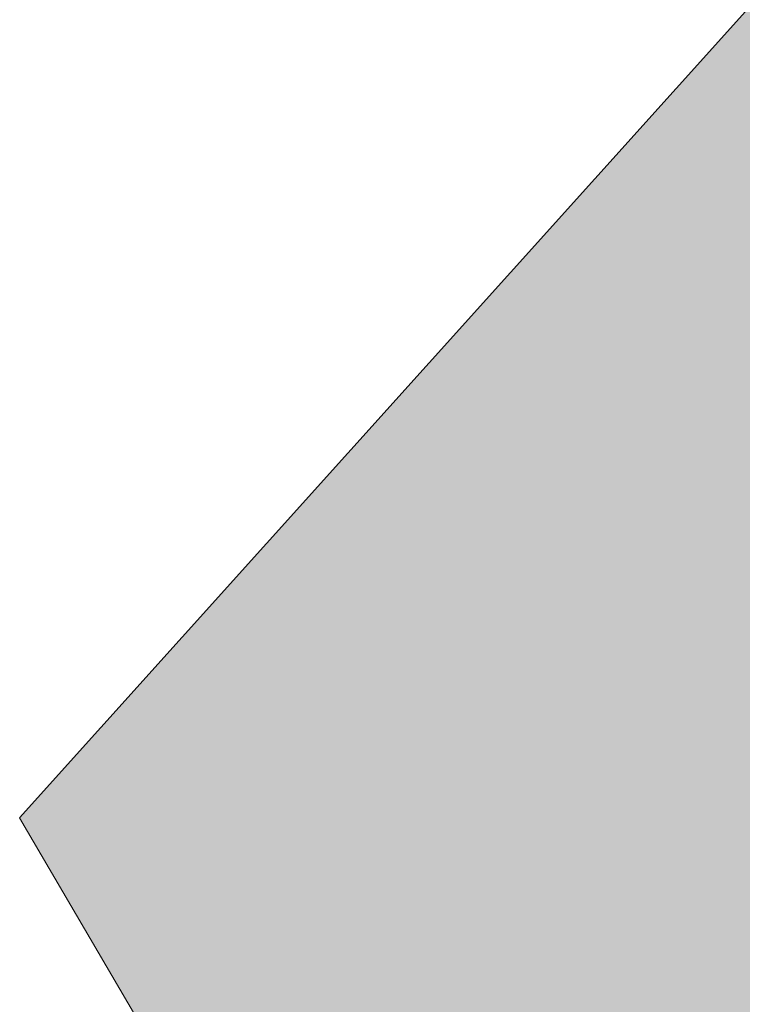
# Model space of a CAD drawing. Units: inches. Extents: x 2091 to 2899, y 967 to 2217.
# Tile 244 of 256: x 2212.563 to 2213.361, y 1135.592 to 1136.679. Entities that reach past the tile are written whole.
import ezdxf

# ---------------------------------------------------------------- set-up
doc = ezdxf.new("R2010")
doc.units = ezdxf.units.IN
doc.layers.add('L-PLNT-PATT', color=114, linetype='Continuous', lineweight=13, true_color=0x139b48)
doc.layers.add('L-PLNT-TREE', color=94, linetype='Continuous', lineweight=13)

# ---------------------------------------------------------------- blocks, each defined once
blk = doc.blocks.new('*U25')
blk.add_lwpolyline([(-1139.42368, 1783.79628), (-1216.11644, 1685.47796), (-1117.5111, 1601.2033), (-1051.7759, 1643.3419), (-1126.09884, 1521.20092), (-1072.10606, 1527.49758), (-1079.90386, 1416.93646), (-1259.93906, 1179.83508), (-1479.05978, 1165.78888), (-1577.66258, 1109.60662), (-1742.00312, 927.01364), (-1676.26538, 814.64658), (-1270.89408, 828.69278), (-1194.20386, 772.51052), (-1007.95074, 856.78518), (-876.4778, 575.87134), (-821.70016, 575.87134), (-569.71184, 884.87504)])

msp = doc.modelspace()

# ---------------------------------------------------------------- hatches: boundary and pattern name
at = {"layer": 'L-PLNT-PATT'}
h = msp.add_hatch(color=256, dxfattribs=at)
h.dxf.hatch_style = 1
h.paths.add_polyline_path([(2333.3376, 1165.6587), (2329.0242, 1166.2116), (2331.6122, 1168.4235), (2335.0629, 1177.2712), (2328.1615, 1184.4599), (2319.5348, 1187.2248), (2323.4168, 1193.3076), (2319.9661, 1203.8142), (2317.8094, 1203.8142), (2313.496, 1213.2148), (2310.908, 1212.6618), (2307.8887, 1212.6618), (2305.7319, 1217.0857), (2307.0259, 1223.1684), (2310.4767, 1223.1684), (2304.0066, 1230.9101), (2303.1363, 1237.0465), (2299.6932, 1240.8637), (2296.6739, 1237.5459), (2294.9485, 1238.6518), (2294.5171, 1241.4166), (2292.3605, 1242.5227), (2289.3411, 1239.7577), (2285.8904, 1240.3107), (2283.3024, 1235.3339), (2283.3024, 1230.9101), (2286.7531, 1229.2512), (2284.165, 1227.5922), (2281.577, 1229.8042), (2274.2442, 1222.6154), (2274.2442, 1220.9565), (2271.2249, 1219.2976), (2272.0876, 1217.6386), (2274.2442, 1214.3208), (2270.3622, 1211.5559), (2266.4801, 1214.3208), (2264.3235, 1213.7678), (2263.4608, 1211.5559), (2266.4801, 1211.0029), (2266.9115, 1206.5791), (2263.5392, 1207.132), (2259.5788, 1203.2612), (2263.8921, 1202.7082), (2262.1668, 1197.1784), (2258.2848, 1196.6254), (2253.9714, 1193.8606), (2248.7953, 1191.0957), (2248.364, 1193.3076), (2244.4819, 1185.0129), (2251.3833, 1186.6718), (2255.6967, 1183.9069), (2254.4027, 1177.2712), (2246.6387, 1174.5063), (2243.1879, 1176.7182), (2241.8939, 1173.4003), (2238.8746, 1172.8474), (2236.2865, 1169.5295), (2233.2671, 1165.6587), (2237.1492, 1162.3408), (2239.7372, 1163.9998), (2236.8111, 1159.1911), (2238.9368, 1159.439), (2238.6298, 1155.0862), (2231.5418, 1145.7515), (2222.915, 1145.1985), (2219.033, 1142.9866), (2212.5629, 1135.7979), (2215.151, 1131.374), (2231.1105, 1131.927), (2234.1298, 1129.7151), (2241.4626, 1133.033), (2246.6387, 1121.9734), (2248.7953, 1121.9734), (2258.7161, 1134.1389), (2261.7355, 1135.7979), (2263.8921, 1133.033), (2263.8921, 1129.1621), (2267.3429, 1128.0562), (2272.0876, 1128.0562), (2273.8129, 1131.927), (2279.4203, 1134.6919), (2285.0278, 1135.2449), (2287.6158, 1137.4568), (2288.0471, 1138.0098), (2289.3411, 1140.7747), (2291.0665, 1139.6687), (2292.3605, 1135.2449), (2295.3798, 1136.9038), (2296.2425, 1135.7979), (2297.1052, 1133.033), (2300.1246, 1138.0098), (2303.1439, 1138.0098), (2304.4379, 1135.7979), (2303.1439, 1133.586), (2306.5946, 1134.6919), (2307.8887, 1133.033), (2310.908, 1135.2449), (2313.9274, 1134.1389), (2319.9661, 1128.0562), (2322.5541, 1126.9502), (2324.7108, 1124.7383), (2342.827, 1126.3972), (2346.2777, 1123.0794), (2348.8658, 1124.1853), (2341.9643, 1133.033), (2341.533, 1136.3508), (2343.6897, 1139.6687), (2339.8077, 1150.1753), (2337.651, 1150.1753)])
h.paths.add_polyline_path([(2339.6578, 1120.6164), (2337.9038, 1120.3574), (2338.4438, 1119.5784), (2340.3328, 1119.6654)])
h.paths.add_polyline_path([(2341.1428, 1118.5404), (2339.0508, 1118.6264), (2339.0508, 1117.6754), (2340.9408, 1116.9824)])
h.paths.add_polyline_path([(2336.5538, 1120.8764), (2335.2038, 1120.3574), (2334.7988, 1118.9724), (2336.8238, 1119.5784)])
h.paths.add_polyline_path([(2337.2958, 1118.9724), (2336.6208, 1118.2804), (2337.6338, 1117.7614)])
h.paths.add_polyline_path([(2338.6458, 1118.7134), (2339.1858, 1119.3194), (2338.2408, 1118.8864), (2338.2408, 1118.1074)])
h.paths.add_polyline_path([(2339.0508, 1122.8664), (2337.7688, 1123.8184), (2337.0938, 1123.1254), (2337.2958, 1121.8284)])
h.paths.add_polyline_path([(2341.6148, 1122.0014), (2341.1428, 1121.8284), (2340.6708, 1122.9524), (2340.1308, 1121.8284), (2340.5358, 1121.0494), (2341.7498, 1120.5304), (2342.8298, 1121.2224)])
h.paths.add_polyline_path([(2342.9648, 1119.7514), (2342.0198, 1119.4914), (2342.0878, 1118.0214), (2343.0328, 1118.4534)])
h.paths.add_polyline_path([(2345.8668, 1118.1944), (2344.3828, 1118.6264), (2343.7078, 1118.0214), (2345.5298, 1117.3294)])
h.paths.add_polyline_path([(2344.6518, 1116.8094), (2343.6398, 1116.4634), (2343.0328, 1115.9444), (2343.9098, 1114.9064), (2344.6518, 1115.3394), (2344.1798, 1115.6854)])
h.paths.add_polyline_path([(2346.8118, 1116.9824), (2345.7318, 1115.8584), (2345.5298, 1114.1274), (2347.0138, 1112.3104), (2348.2968, 1112.2244), (2346.8798, 1114.3004), (2345.8668, 1114.2144), (2346.8118, 1114.6464)])
h.paths.add_polyline_path([(2345.2598, 1116.5504), (2344.7198, 1116.3774), (2344.9218, 1115.6854), (2345.1248, 1115.8584)])
h.paths.add_polyline_path([(2342.6948, 1116.8964), (2342.0198, 1117.3294), (2341.9528, 1116.6364)])
h.paths.add_polyline_path([(2341.4808, 1120.0974), (2341.1428, 1120.0974), (2341.0758, 1119.5784), (2341.4808, 1119.4054)])
h.paths.add_polyline_path([(2343.9778, 1121.1354), (2343.6398, 1119.7514), (2345.0568, 1119.7514)])
h.paths.add_polyline_path([(2339.1178, 1121.7414), (2338.3758, 1121.5684), (2338.1738, 1121.0494), (2338.8478, 1121.2224)])
h.paths.add_polyline_path([(2336.3508, 1122.4334), (2335.7438, 1122.7794), (2334.5288, 1123.4714), (2334.9338, 1122.4334), (2336.0138, 1121.9144)])
h.paths.add_polyline_path([(2334.4618, 1122.1744), (2332.0998, 1122.8664), (2331.3568, 1122.1744), (2332.5718, 1121.3084)])
h.paths.add_polyline_path([(2334.5968, 1121.3084), (2334.0568, 1120.7894), (2334.2588, 1120.3574), (2334.7318, 1120.8764)])
h.paths.add_polyline_path([(2332.5048, 1120.7894), (2331.6948, 1120.4434), (2332.7068, 1119.6654)])
h.paths.add_polyline_path([(2333.6518, 1119.3194), (2333.3818, 1118.4534), (2334.2588, 1118.5404)])
h.paths.add_polyline_path([(2331.9648, 1118.1944), (2331.0868, 1116.2904), (2332.6398, 1116.6364)])
h.paths.add_polyline_path([(2330.7498, 1121.5684), (2328.9948, 1121.0494), (2328.5228, 1119.3194), (2330.2768, 1120.2704)])
h.paths.add_polyline_path([(2330.7498, 1118.6264), (2329.8728, 1118.0214), (2330.0078, 1117.5024)])
h.paths.add_polyline_path([(2328.3878, 1117.8484), (2327.1728, 1117.7614), (2327.5098, 1116.5504)])
h.paths.add_polyline_path([(2326.9028, 1115.2524), (2326.0928, 1115.3394), (2325.2158, 1113.6084), (2326.7008, 1114.1274)])
h.paths.add_polyline_path([(2328.6578, 1114.3874), (2328.3198, 1114.9064), (2328.0498, 1114.1274)])
h.paths.add_polyline_path([(2326.7008, 1112.6564), (2327.1058, 1112.1374), (2328.3198, 1112.2244)])
h.paths.add_polyline_path([(2329.5348, 1113.6084), (2328.5898, 1113.3494), (2329.0628, 1112.3104)])
h.paths.add_polyline_path([(2340.3328, 1115.3394), (2339.3878, 1115.3394), (2340.0628, 1113.6954)])
h.paths.add_polyline_path([(2340.9408, 1116.3774), (2340.8058, 1115.5124), (2342.0198, 1115.0794)])
h.paths.add_polyline_path([(2341.8178, 1114.4734), (2340.8058, 1114.5604), (2340.9408, 1113.0894)])
h.paths.add_polyline_path([(2343.0328, 1112.2244), (2342.3578, 1113.3494), (2341.5478, 1112.2244), (2342.0198, 1111.7914)])
h.paths.add_polyline_path([(2342.7628, 1113.9544), (2343.4378, 1113.0894), (2344.0448, 1113.5224)])
h.paths.add_polyline_path([(2344.7198, 1114.3874), (2344.4498, 1113.8684), (2345.1918, 1113.3494)])
h.paths.add_polyline_path([(2345.6648, 1112.3104), (2344.6518, 1112.5704), (2344.0448, 1111.9644), (2345.4618, 1111.5324)])
h.paths.add_polyline_path([(2344.3148, 1111.0124), (2342.9648, 1111.0994), (2342.9648, 1110.3204)])
h.paths.add_polyline_path([(2344.8548, 1110.0614), (2344.1128, 1109.7154), (2344.5168, 1109.2824)])
h.paths.add_polyline_path([(2346.6768, 1109.2824), (2345.8668, 1110.0614), (2346.0698, 1108.0714)])
h.paths.add_polyline_path([(2347.0138, 1110.9264), (2346.6098, 1111.1864), (2346.2718, 1110.4934)])
h.paths.add_polyline_path([(2345.8668, 1106.6864), (2344.5168, 1106.6004), (2344.9898, 1105.5624)])
h.paths.add_polyline_path([(2345.1248, 1104.6974), (2344.4498, 1104.2644), (2344.5848, 1103.7454)])
h.paths.add_polyline_path([(2343.7748, 1104.4374), (2343.4378, 1105.1294), (2342.6948, 1104.6104), (2342.6278, 1102.8804)])
h.paths.add_polyline_path([(2341.8178, 1103.8314), (2341.1428, 1103.6584), (2341.5478, 1102.8804)])
h.paths.add_polyline_path([(2342.5598, 1102.3614), (2341.9528, 1101.8414), (2342.6948, 1101.6684)])
h.paths.add_polyline_path([(2341.1428, 1101.9284), (2340.6028, 1102.3614), (2340.0628, 1101.8414), (2340.6028, 1101.2364)])
h.paths.add_polyline_path([(2336.7558, 1101.2364), (2337.3638, 1100.5434), (2339.1178, 1100.4574)])
h.paths.add_polyline_path([(2335.2718, 1103.3124), (2334.1918, 1102.6204), (2335.5418, 1102.2744)])
h.paths.add_polyline_path([(2333.9888, 1101.7554), (2333.5168, 1101.5824), (2334.7318, 1101.1494)])
h.paths.add_polyline_path([(2331.6948, 1102.9664), (2330.5468, 1102.0144), (2332.0998, 1102.3614)])
h.paths.add_polyline_path([(2329.7378, 1106.5134), (2328.2528, 1106.0814), (2329.5348, 1105.3024)])
h.paths.add_polyline_path([(2326.6328, 1108.3304), (2326.4978, 1109.1094), (2325.8908, 1108.5034), (2326.0928, 1107.3794)])
h.paths.add_polyline_path([(2240.5961, 1257.8142), (2239.5841, 1257.4682), (2238.9771, 1256.9492), (2239.8541, 1255.9112), (2240.5961, 1256.3442), (2240.1241, 1256.6902)])
h.paths.add_polyline_path([(2241.8111, 1259.1992), (2240.3271, 1259.6312), (2239.6521, 1259.0262), (2241.4741, 1258.3342)])
h.paths.add_polyline_path([(2242.7561, 1257.9872), (2241.6761, 1256.8632), (2241.4741, 1255.1322), (2242.9581, 1253.3152), (2244.2411, 1253.2292), (2242.8241, 1255.3052), (2241.8111, 1255.2192), (2242.7561, 1255.6512)])
h.paths.add_polyline_path([(2241.6091, 1253.3152), (2240.5961, 1253.5752), (2239.9891, 1252.9692), (2241.4061, 1252.5372)])
h.paths.add_polyline_path([(2240.6641, 1255.3922), (2240.3941, 1254.8732), (2241.1361, 1254.3542)])
h.paths.add_polyline_path([(2242.9581, 1251.9312), (2242.5541, 1252.1912), (2242.2161, 1251.4982)])
h.paths.add_polyline_path([(2240.2591, 1252.0172), (2238.9091, 1252.1042), (2238.9091, 1251.3252)])
h.paths.add_polyline_path([(2238.3021, 1254.3542), (2237.4921, 1253.2292), (2237.9641, 1252.7962), (2238.9771, 1253.2292)])
h.paths.add_polyline_path([(2239.9891, 1254.5272), (2238.7071, 1254.9592), (2239.3821, 1254.0942)])
h.paths.add_polyline_path([(2240.7991, 1251.0662), (2240.0571, 1250.7202), (2240.4611, 1250.2872)])
h.paths.add_polyline_path([(2241.8111, 1251.0662), (2242.0141, 1249.0762), (2242.6211, 1250.2872)])
h.paths.add_polyline_path([(2241.2041, 1257.5552), (2240.6641, 1257.3822), (2240.8661, 1256.6902), (2241.0691, 1256.8632)])
h.paths.add_polyline_path([(2238.6391, 1257.9012), (2237.9641, 1258.3342), (2237.8971, 1257.6412)])
h.paths.add_polyline_path([(2238.9091, 1260.7562), (2237.9641, 1260.4962), (2238.0321, 1259.0262), (2238.9771, 1259.4582)])
h.paths.add_polyline_path([(2239.9221, 1262.1402), (2239.5841, 1260.7562), (2241.0011, 1260.7562)])
h.paths.add_polyline_path([(2238.7741, 1262.2272), (2237.5591, 1263.0062), (2237.0871, 1262.8332), (2236.6151, 1263.9572), (2236.0751, 1262.8332), (2236.4801, 1262.0542), (2237.6941, 1261.5352)])
h.paths.add_polyline_path([(2237.4251, 1261.1022), (2237.0871, 1261.1022), (2237.0201, 1260.5832), (2237.4251, 1260.4102)])
h.paths.add_polyline_path([(2237.0871, 1259.5452), (2234.9951, 1259.6312), (2234.9951, 1258.6802), (2236.8851, 1257.9872)])
h.paths.add_polyline_path([(2236.8851, 1257.3822), (2236.7501, 1256.5172), (2237.9641, 1256.0842)])
h.paths.add_polyline_path([(2237.7621, 1255.4782), (2236.7501, 1255.5652), (2236.8851, 1254.0942)])
h.paths.add_polyline_path([(2236.2771, 1256.3442), (2235.3321, 1256.3442), (2236.0071, 1254.7002)])
h.paths.add_polyline_path([(2241.8111, 1247.6912), (2240.4611, 1247.6052), (2240.9341, 1246.5672)])
h.paths.add_polyline_path([(2239.7191, 1245.4422), (2239.3821, 1246.1342), (2238.6391, 1245.6152), (2238.5721, 1243.8852)])
h.paths.add_polyline_path([(2241.0691, 1245.7022), (2240.3941, 1245.2692), (2240.5291, 1244.7502)])
h.paths.add_polyline_path([(2237.7621, 1244.8362), (2237.0871, 1244.6632), (2237.4921, 1243.8852)])
h.paths.add_polyline_path([(2237.0871, 1242.9332), (2236.5471, 1243.3662), (2236.0071, 1242.8462), (2236.5471, 1242.2412)])
h.paths.add_polyline_path([(2238.5041, 1243.3662), (2237.8971, 1242.8462), (2238.6391, 1242.6732)])
h.paths.add_polyline_path([(2232.7001, 1242.2412), (2233.3081, 1241.5482), (2235.0621, 1241.4622)], flags=17)
h.paths.add_polyline_path([(2231.2161, 1244.3172), (2230.1361, 1243.6252), (2231.4861, 1243.2792)])
h.paths.add_polyline_path([(2229.9331, 1242.7602), (2229.4611, 1242.5872), (2230.6761, 1242.1542)])
h.paths.add_polyline_path([(2227.6391, 1243.9712), (2226.4911, 1243.0192), (2228.0441, 1243.3662)])
h.paths.add_polyline_path([(2222.5771, 1249.3352), (2222.4421, 1250.1142), (2221.8351, 1249.5082), (2222.0371, 1248.3842)])
h.paths.add_polyline_path([(2225.6821, 1247.5182), (2224.1971, 1247.0862), (2225.4791, 1246.3072)])
h.paths.add_polyline_path([(2225.4791, 1254.6132), (2224.5341, 1254.3542), (2225.0071, 1253.3152)])
h.paths.add_polyline_path([(2224.2641, 1253.2292), (2222.6451, 1253.6612), (2223.0501, 1253.1422)])
h.paths.add_polyline_path([(2222.8471, 1256.2572), (2222.0371, 1256.3442), (2221.1601, 1254.6132), (2222.6451, 1255.1322)])
h.paths.add_polyline_path([(2224.3321, 1258.8532), (2223.1171, 1258.7662), (2223.4541, 1257.5552)])
h.paths.add_polyline_path([(2226.6941, 1259.6312), (2225.8171, 1259.0262), (2225.9521, 1258.5072)])
h.paths.add_polyline_path([(2227.9091, 1259.1992), (2227.0311, 1257.2952), (2228.5841, 1257.6412)])
h.paths.add_polyline_path([(2224.2641, 1255.9112), (2223.9941, 1255.1322), (2224.6021, 1255.3922)])
h.paths.add_polyline_path([(2229.5961, 1260.3242), (2229.3261, 1259.4582), (2230.2031, 1259.5452)])
h.paths.add_polyline_path([(2228.4491, 1261.7942), (2227.6391, 1261.4482), (2228.6511, 1260.6702)])
h.paths.add_polyline_path([(2230.4061, 1263.1792), (2228.0441, 1263.8712), (2227.3011, 1263.1792), (2228.5161, 1262.3132)])
h.paths.add_polyline_path([(2232.7681, 1260.5832), (2232.4981, 1261.8812), (2231.1481, 1261.3622), (2230.7431, 1259.9772)])
h.paths.add_polyline_path([(2230.6761, 1261.8812), (2230.5411, 1262.3132), (2230.0011, 1261.7942), (2230.2031, 1261.3622)])
h.paths.add_polyline_path([(2232.2951, 1263.4382), (2231.6881, 1263.7842), (2230.4731, 1264.4762), (2230.8781, 1263.4382), (2231.9581, 1262.9192)])
h.paths.add_polyline_path([(2234.9951, 1263.8712), (2233.7131, 1264.8232), (2233.0381, 1264.1302), (2233.2401, 1262.8332)])
h.paths.add_polyline_path([(2235.0621, 1262.7462), (2234.3201, 1262.5732), (2234.1181, 1262.0542), (2234.7921, 1262.2272)])
h.paths.add_polyline_path([(2235.6021, 1261.6212), (2233.8481, 1261.3622), (2234.3881, 1260.5832), (2236.2771, 1260.6702)])
h.paths.add_polyline_path([(2235.1301, 1260.3242), (2234.1851, 1259.8912), (2234.1851, 1259.1122), (2234.5901, 1259.7182)])
h.paths.add_polyline_path([(2226.6941, 1262.5732), (2224.9391, 1262.0542), (2224.4671, 1260.3242), (2226.2211, 1261.2752)])
h.paths.add_polyline_path([(2233.2401, 1259.9772), (2232.5651, 1259.2852), (2233.5781, 1258.7662)])
h.paths.add_polyline_path([(2337.2674, 1337.8275), (2336.1874, 1336.7035), (2335.9854, 1334.9725), (2337.4694, 1333.1555), (2338.7524, 1333.0695), (2337.3354, 1335.1455), (2336.3224, 1335.0595), (2337.2674, 1335.4915)])
h.paths.add_polyline_path([(2336.3224, 1339.0395), (2334.8384, 1339.4715), (2334.1634, 1338.8665), (2335.9854, 1338.1745)])
h.paths.add_polyline_path([(2334.4334, 1341.9805), (2334.0954, 1340.5965), (2335.5124, 1340.5965)])
h.paths.add_polyline_path([(2333.2854, 1342.0675), (2332.0704, 1342.8465), (2331.5984, 1342.6735), (2331.1264, 1343.7975), (2330.5864, 1342.6735), (2330.9914, 1341.8945), (2332.2054, 1341.3755)])
h.paths.add_polyline_path([(2333.4204, 1340.5965), (2332.4754, 1340.3365), (2332.5434, 1338.8665), (2333.4884, 1339.2985)])
h.paths.add_polyline_path([(2331.9364, 1340.9425), (2331.5984, 1340.9425), (2331.5314, 1340.4235), (2331.9364, 1340.2505)])
h.paths.add_polyline_path([(2329.5734, 1342.5865), (2328.8314, 1342.4135), (2328.6294, 1341.8945), (2329.3034, 1342.0675)])
h.paths.add_polyline_path([(2329.5064, 1343.7115), (2328.2244, 1344.6635), (2327.5494, 1343.9705), (2327.7514, 1342.6735)])
h.paths.add_polyline_path([(2330.1134, 1341.4615), (2328.3594, 1341.2025), (2328.8994, 1340.4235), (2330.7884, 1340.5105)])
h.paths.add_polyline_path([(2331.5984, 1339.3855), (2329.5064, 1339.4715), (2329.5064, 1338.5205), (2331.3964, 1337.8275)])
h.paths.add_polyline_path([(2327.0094, 1341.7215), (2325.6594, 1341.2025), (2325.2544, 1339.8175), (2327.2794, 1340.4235)])
h.paths.add_polyline_path([(2326.8064, 1343.2785), (2326.1994, 1343.6245), (2324.9844, 1344.3165), (2325.3894, 1343.2785), (2326.4694, 1342.7595)])
h.paths.add_polyline_path([(2324.9174, 1343.0195), (2322.5554, 1343.7115), (2321.8124, 1343.0195), (2323.0274, 1342.1535)])
h.paths.add_polyline_path([(2321.2054, 1342.4135), (2319.4504, 1341.8945), (2318.9784, 1340.1645), (2320.7324, 1341.1155)])
h.paths.add_polyline_path([(2318.8434, 1338.6935), (2317.6284, 1338.6065), (2317.9654, 1337.3955)])
h.paths.add_polyline_path([(2322.4204, 1339.0395), (2321.5424, 1337.1355), (2323.0954, 1337.4815)])
h.paths.add_polyline_path([(2324.1074, 1340.1645), (2323.8374, 1339.2985), (2324.7144, 1339.3855)])
h.paths.add_polyline_path([(2322.9604, 1341.6345), (2322.1504, 1341.2885), (2323.1624, 1340.5105)])
h.paths.add_polyline_path([(2325.1874, 1341.7215), (2325.0524, 1342.1535), (2324.5124, 1341.6345), (2324.7144, 1341.2025)])
h.paths.add_polyline_path([(2321.2054, 1339.4715), (2320.3284, 1338.8665), (2320.4634, 1338.3475)])
h.paths.add_polyline_path([(2317.3584, 1336.0975), (2316.5484, 1336.1845), (2315.6714, 1334.4535), (2317.1564, 1334.9725)])
h.paths.add_polyline_path([(2318.7754, 1335.7515), (2318.5054, 1334.9725), (2319.1134, 1335.2325)])
h.paths.add_polyline_path([(2319.9904, 1334.4535), (2319.0454, 1334.1945), (2319.5184, 1333.1555)])
h.paths.add_polyline_path([(2317.1564, 1333.5015), (2317.5614, 1332.9825), (2318.7754, 1333.0695)])
h.paths.add_polyline_path([(2317.0884, 1329.1755), (2316.9534, 1329.9545), (2316.3464, 1329.3485), (2316.5484, 1328.2245)])
h.paths.add_polyline_path([(2320.1934, 1327.3585), (2318.7084, 1326.9265), (2319.9904, 1326.1475)])
h.paths.add_polyline_path([(2322.1504, 1323.8115), (2321.0024, 1322.8595), (2322.5554, 1323.2065)])
h.paths.add_polyline_path([(2325.7274, 1324.1575), (2324.6474, 1323.4655), (2325.9974, 1323.1195)])
h.paths.add_polyline_path([(2334.2304, 1325.2825), (2333.8934, 1325.9745), (2333.1504, 1325.4555), (2333.0834, 1323.7255)])
h.paths.add_polyline_path([(2336.3224, 1327.5315), (2334.9724, 1327.4455), (2335.4454, 1326.4075)])
h.paths.add_polyline_path([(2335.3104, 1330.9065), (2334.5684, 1330.5605), (2334.9724, 1330.1275)])
h.paths.add_polyline_path([(2334.7704, 1331.8575), (2333.4204, 1331.9445), (2333.4204, 1331.1655)])
h.paths.add_polyline_path([(2332.8134, 1334.1945), (2332.0034, 1333.0695), (2332.4754, 1332.6365), (2333.4884, 1333.0695)])
h.paths.add_polyline_path([(2335.1074, 1333.4155), (2334.5004, 1332.8095), (2335.9174, 1332.3775), (2336.1204, 1333.1555)])
h.paths.add_polyline_path([(2334.6354, 1336.5305), (2335.1074, 1337.6545), (2334.0954, 1337.3085), (2333.4884, 1336.7895), (2334.3654, 1335.7515), (2335.1074, 1336.1845)])
h.paths.add_polyline_path([(2335.7154, 1337.3955), (2335.1754, 1337.2225), (2335.3774, 1336.5305), (2335.5804, 1336.7035)])
h.paths.add_polyline_path([(2333.1504, 1337.7415), (2332.4754, 1338.1745), (2332.4084, 1337.4815)])
h.paths.add_polyline_path([(2330.7884, 1336.1845), (2329.8434, 1336.1845), (2330.5184, 1334.5405)])
h.paths.add_polyline_path([(2332.2734, 1335.3185), (2331.2614, 1335.4055), (2331.3964, 1333.9345)])
h.paths.add_polyline_path([(2331.3964, 1337.2225), (2331.2614, 1336.3575), (2332.4754, 1335.9245)])
h.paths.add_polyline_path([(2334.5004, 1334.3675), (2333.2184, 1334.7995), (2333.8934, 1333.9345)])
h.paths.add_polyline_path([(2335.1754, 1335.2325), (2334.9054, 1334.7135), (2335.6474, 1334.1945)])
h.paths.add_polyline_path([(2337.1324, 1330.1275), (2336.3224, 1330.9065), (2336.5254, 1328.9165)])
h.paths.add_polyline_path([(2337.0654, 1332.0315), (2336.7274, 1331.3385), (2337.4694, 1331.7715)])
h.paths.add_polyline_path([(2329.6414, 1340.1645), (2328.6964, 1339.7315), (2328.6964, 1338.9525), (2329.1014, 1339.5585)])
h.paths.add_polyline_path([(2327.7514, 1339.8175), (2327.0764, 1339.1255), (2328.0894, 1338.6065)])
h.paths.add_polyline_path([(2327.2114, 1322.0815), (2327.8194, 1321.3885), (2329.5734, 1321.3025)])
h.paths.add_polyline_path([(2324.4444, 1322.6005), (2323.9724, 1322.4275), (2325.1874, 1321.9945)])
h.paths.add_polyline_path([(2331.0584, 1323.2065), (2330.5184, 1322.6865), (2331.0584, 1322.0815), (2331.5984, 1322.7735)])
h.paths.add_polyline_path([(2332.2734, 1324.6765), (2331.5984, 1324.5035), (2332.0034, 1323.7255)])
h.paths.add_polyline_path([(2333.0154, 1323.2065), (2332.4084, 1322.6865), (2333.1504, 1322.5135)])
h.paths.add_polyline_path([(2335.5804, 1325.5425), (2334.9054, 1325.1095), (2335.0404, 1324.5905)])
h.paths.add_polyline_path([(2271.0827, 1964.3172), (2776.853, 1964.3172), (2776.853, 2037.1696), (2271.0827, 2037.1696)], flags=9)
h.paths.add_polyline_path([(2380.6493, 1536.8241), (2461.0408, 1536.8241), (2461.0408, 1554.6526), (2380.6493, 1554.6526)], flags=9)
h.paths.add_polyline_path([(2240.7557, 1609.7255), (2309.1858, 1609.7255), (2309.1858, 1617.6982), (2240.7557, 1617.6982)], flags=9)
h.paths.add_polyline_path([(2212.6773, 1313.5041), (2282.5915, 1313.5041), (2282.5915, 1322.7452), (2212.6773, 1322.7452)], flags=9)
h.paths.add_polyline_path([(2457.112, 1114.7786), (2558.4816, 1114.7786), (2558.4816, 1142.2197), (2457.112, 1142.2197)], flags=9)
h.paths.add_polyline_path([(2473.4423, 1273.0101), (2604.6412, 1273.0101), (2604.6412, 1318.3469), (2473.4423, 1318.3469)], flags=9)
h.paths.add_polyline_path([(2638.8763, 1626.9774), (2684.2504, 1627.9767), (2684.0385, 1637.5975), (2638.6644, 1636.5982)], flags=9)
h.paths.add_polyline_path([(2537.5906, 1453.7934), (2628.3895, 1453.7934), (2628.3895, 1475.3448), (2537.5906, 1475.3448)], flags=9)
h.paths.add_polyline_path([(2504.1376, 1714.6324), (2554.6472, 1714.6324), (2554.6472, 1730.2377), (2504.1376, 1730.2377)], flags=9)
h.paths.add_polyline_path([(2487.5012, 1575.6519), (2535.0971, 1575.6519), (2535.0971, 1598.3776), (2487.5012, 1598.3776)], flags=9)
h.paths.add_polyline_path([(2709.0994, 1735.7103), (2740.0166, 1735.7103), (2740.0166, 1749.9376), (2709.0994, 1749.9376)], flags=9)
h.paths.add_polyline_path([(2442.4384, 1792.1717), (2564.7288, 1792.1717), (2564.7288, 1842.0002), (2442.4384, 1842.0002)], flags=9)
h.paths.add_polyline_path([(2655.8158, 1809.6441), (2789.5201, 1806.6938), (2790.085, 1832.2916), (2656.3806, 1835.2419)], flags=9)
h.paths.add_polyline_path([(2234.8427, 1797.7201), (2368.5929, 1794.7689), (2369.1607, 1820.5041), (2235.4106, 1823.4554)], flags=9)
h.paths.add_polyline_path([(2245.1385, 1644.0063), (2398.4277, 1640.6239), (2398.9948, 1666.3248), (2245.7056, 1669.7073)], flags=9)
h.paths.add_polyline_path([(2306.1428, 1431.1685), (2413.7683, 1428.7937), (2414.3331, 1454.3915), (2306.7077, 1456.7664)], flags=9)
h.paths.add_polyline_path([(2306.8346, 1458.2331), (2393.3805, 1456.3234), (2393.9328, 1481.3544), (2307.3869, 1483.2641)], flags=9)

# ---------------------------------------------------------------- block references
at = {"layer": 'L-PLNT-TREE', "xscale": 0.0393700787401575, "yscale": 0.0393700787401575, "zscale": 0.0393700787401575}
msp.add_blockref('*U25', (2281.1457, 1099.3013), dxfattribs=at)

doc.saveas('drawing.dxf')
